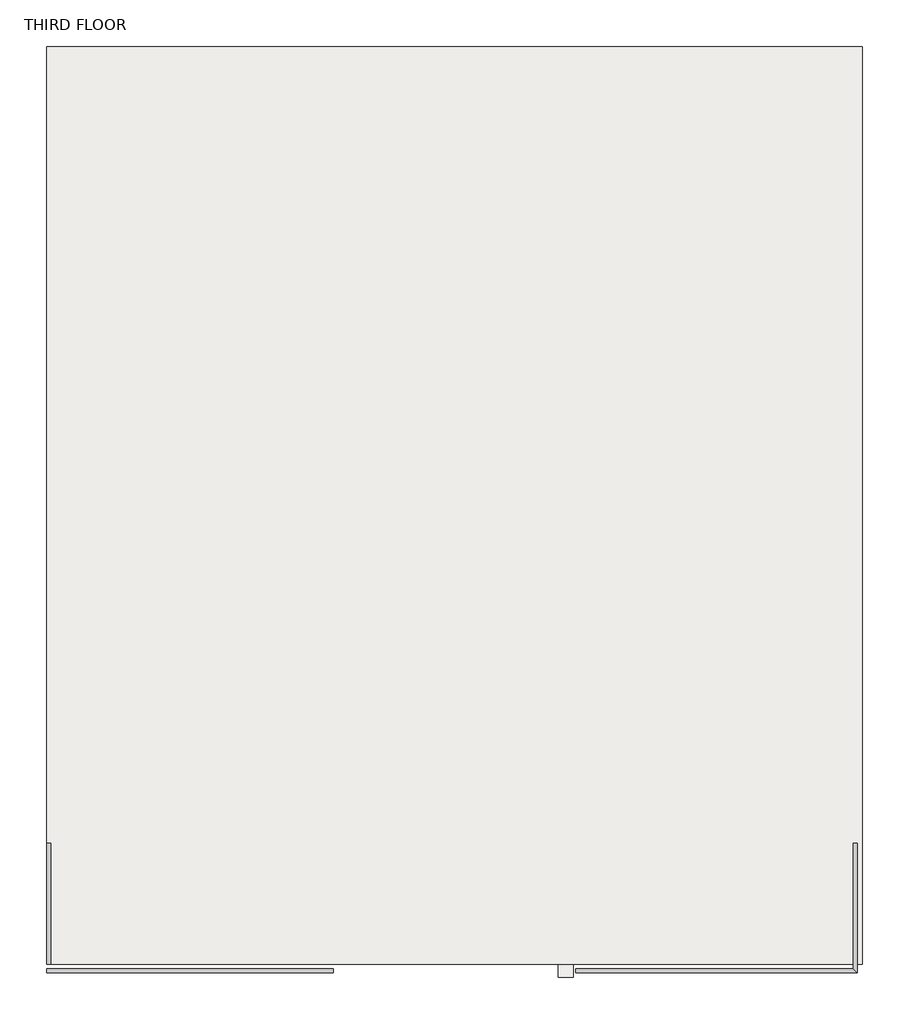
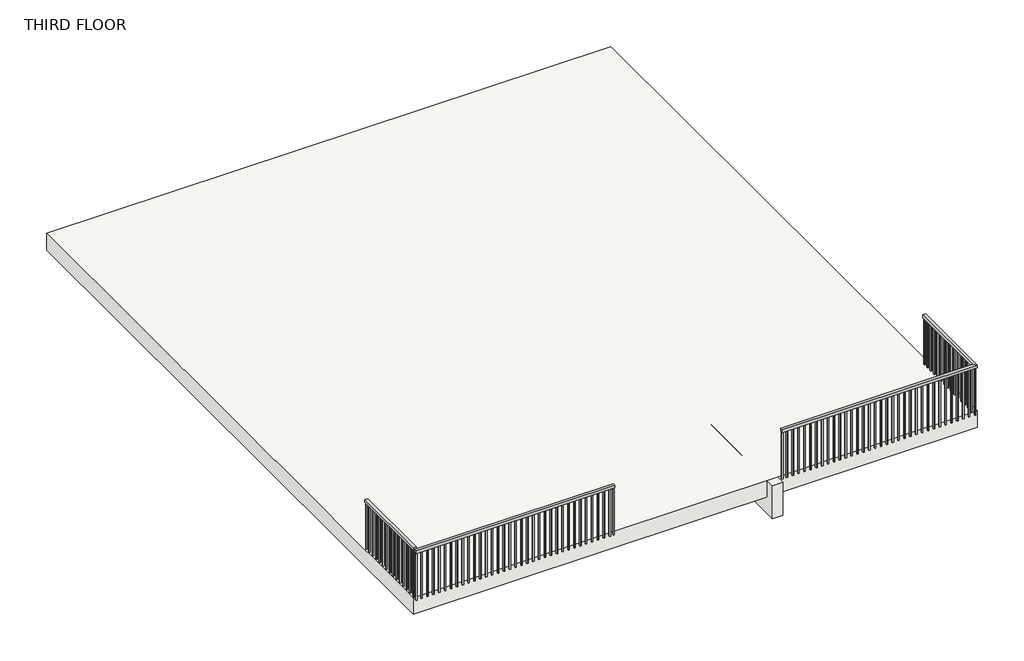
# One storey: 3 railings, 2 slabs.
"""IFC4 building model written with IfcOpenShell, lengths in millimetres."""

from ifc_helpers import new_model, si_unit, frame, origin, place, context, project, spatial, polyline, outline, extrude, faceted_brep, transform, mapped, element, save
from components import floors_4_floors_3_d07f1cc1

model = new_model("IFC4")

# Units and contexts
model_context = context("Model", 3, world=origin())
ifc_project = project(units=[si_unit("LENGTHUNIT", "METRE", prefix="MILLI")], contexts=[model_context])

# Site, building, storey
site = spatial("IfcSite", under=ifc_project)
building = spatial("IfcBuilding", under=site)
storey = spatial("IfcBuildingStorey", under=building, Name="THIRD FLOOR", Elevation=9144.0)

# Railings
placement = place(None, origin())
element("IfcRailing", 1, ObjectType="Handrail - Rectangular", at=placement, inside=storey, context=model_context, shape_type="SweptSolid", body=[
    extrude(outline(polyline([(-6322.0230786, -2172.0464178), (-6322.0230786, -2121.2464178), (-2893.0230786, -2121.2464178), (-2893.0230786, -2172.0464178), (-6322.0230786, -2172.0464178)])), frame((0.0, 0.0, 10007.6), z_axis=(0.0, 0.0, 1.0), x_axis=(1.0, 0.0, 0.0)), (0.0, 0.0, 1.0), 50.8),
    extrude(outline(polyline([(-2978.7480786, -2156.1714178), (-2978.7480786, -2137.1214178), (-2959.6980786, -2137.1214178), (-2959.6980786, -2156.1714178), (-2978.7480786, -2156.1714178)])), frame((0.0, 0.0, 9144.0), z_axis=(0.0, 0.0, 1.0), x_axis=(1.0, 0.0, 0.0)), (0.0, 0.0, 1.0), 863.6),
    extrude(outline(polyline([(-3080.3480786, -2156.1714178), (-3080.3480786, -2137.1214178), (-3061.2980786, -2137.1214178), (-3061.2980786, -2156.1714178), (-3080.3480786, -2156.1714178)])), frame((0.0, 0.0, 9144.0), z_axis=(0.0, 0.0, 1.0), x_axis=(1.0, 0.0, 0.0)), (0.0, 0.0, 1.0), 863.6),
    extrude(outline(polyline([(-3181.9480786, -2156.1714178), (-3181.9480786, -2137.1214178), (-3162.8980786, -2137.1214178), (-3162.8980786, -2156.1714178), (-3181.9480786, -2156.1714178)])), frame((0.0, 0.0, 9144.0), z_axis=(0.0, 0.0, 1.0), x_axis=(1.0, 0.0, 0.0)), (0.0, 0.0, 1.0), 863.6),
    extrude(outline(polyline([(-3283.5480786, -2156.1714178), (-3283.5480786, -2137.1214178), (-3264.4980786, -2137.1214178), (-3264.4980786, -2156.1714178), (-3283.5480786, -2156.1714178)])), frame((0.0, 0.0, 9144.0), z_axis=(0.0, 0.0, 1.0), x_axis=(1.0, 0.0, 0.0)), (0.0, 0.0, 1.0), 863.6),
    extrude(outline(polyline([(-3385.1480786, -2156.1714178), (-3385.1480786, -2137.1214178), (-3366.0980786, -2137.1214178), (-3366.0980786, -2156.1714178), (-3385.1480786, -2156.1714178)])), frame((0.0, 0.0, 9144.0), z_axis=(0.0, 0.0, 1.0), x_axis=(1.0, 0.0, 0.0)), (0.0, 0.0, 1.0), 863.6),
    extrude(outline(polyline([(-3486.7480786, -2156.1714178), (-3486.7480786, -2137.1214178), (-3467.6980786, -2137.1214178), (-3467.6980786, -2156.1714178), (-3486.7480786, -2156.1714178)])), frame((0.0, 0.0, 9144.0), z_axis=(0.0, 0.0, 1.0), x_axis=(1.0, 0.0, 0.0)), (0.0, 0.0, 1.0), 863.6),
    extrude(outline(polyline([(-3588.3480786, -2156.1714178), (-3588.3480786, -2137.1214178), (-3569.2980786, -2137.1214178), (-3569.2980786, -2156.1714178), (-3588.3480786, -2156.1714178)])), frame((0.0, 0.0, 9144.0), z_axis=(0.0, 0.0, 1.0), x_axis=(1.0, 0.0, 0.0)), (0.0, 0.0, 1.0), 863.6),
    extrude(outline(polyline([(-3689.9480786, -2156.1714178), (-3689.9480786, -2137.1214178), (-3670.8980786, -2137.1214178), (-3670.8980786, -2156.1714178), (-3689.9480786, -2156.1714178)])), frame((0.0, 0.0, 9144.0), z_axis=(0.0, 0.0, 1.0), x_axis=(1.0, 0.0, 0.0)), (0.0, 0.0, 1.0), 863.6),
    extrude(outline(polyline([(-3791.5480786, -2156.1714178), (-3791.5480786, -2137.1214178), (-3772.4980786, -2137.1214178), (-3772.4980786, -2156.1714178), (-3791.5480786, -2156.1714178)])), frame((0.0, 0.0, 9144.0), z_axis=(0.0, 0.0, 1.0), x_axis=(1.0, 0.0, 0.0)), (0.0, 0.0, 1.0), 863.6),
    extrude(outline(polyline([(-3893.1480786, -2156.1714178), (-3893.1480786, -2137.1214178), (-3874.0980786, -2137.1214178), (-3874.0980786, -2156.1714178), (-3893.1480786, -2156.1714178)])), frame((0.0, 0.0, 9144.0), z_axis=(0.0, 0.0, 1.0), x_axis=(1.0, 0.0, 0.0)), (0.0, 0.0, 1.0), 863.6),
    extrude(outline(polyline([(-3994.7480786, -2156.1714178), (-3994.7480786, -2137.1214178), (-3975.6980786, -2137.1214178), (-3975.6980786, -2156.1714178), (-3994.7480786, -2156.1714178)])), frame((0.0, 0.0, 9144.0), z_axis=(0.0, 0.0, 1.0), x_axis=(1.0, 0.0, 0.0)), (0.0, 0.0, 1.0), 863.6),
    extrude(outline(polyline([(-4096.3480786, -2156.1714178), (-4096.3480786, -2137.1214178), (-4077.2980786, -2137.1214178), (-4077.2980786, -2156.1714178), (-4096.3480786, -2156.1714178)])), frame((0.0, 0.0, 9144.0), z_axis=(0.0, 0.0, 1.0), x_axis=(1.0, 0.0, 0.0)), (0.0, 0.0, 1.0), 863.6),
    extrude(outline(polyline([(-4197.9480786, -2156.1714178), (-4197.9480786, -2137.1214178), (-4178.8980786, -2137.1214178), (-4178.8980786, -2156.1714178), (-4197.9480786, -2156.1714178)])), frame((0.0, 0.0, 9144.0), z_axis=(0.0, 0.0, 1.0), x_axis=(1.0, 0.0, 0.0)), (0.0, 0.0, 1.0), 863.6),
    extrude(outline(polyline([(-4299.5480786, -2156.1714178), (-4299.5480786, -2137.1214178), (-4280.4980786, -2137.1214178), (-4280.4980786, -2156.1714178), (-4299.5480786, -2156.1714178)])), frame((0.0, 0.0, 9144.0), z_axis=(0.0, 0.0, 1.0), x_axis=(1.0, 0.0, 0.0)), (0.0, 0.0, 1.0), 863.6),
    extrude(outline(polyline([(-4401.1480786, -2156.1714178), (-4401.1480786, -2137.1214178), (-4382.0980786, -2137.1214178), (-4382.0980786, -2156.1714178), (-4401.1480786, -2156.1714178)])), frame((0.0, 0.0, 9144.0), z_axis=(0.0, 0.0, 1.0), x_axis=(1.0, 0.0, 0.0)), (0.0, 0.0, 1.0), 863.6),
    extrude(outline(polyline([(-4502.7480786, -2156.1714178), (-4502.7480786, -2137.1214178), (-4483.6980786, -2137.1214178), (-4483.6980786, -2156.1714178), (-4502.7480786, -2156.1714178)])), frame((0.0, 0.0, 9144.0), z_axis=(0.0, 0.0, 1.0), x_axis=(1.0, 0.0, 0.0)), (0.0, 0.0, 1.0), 863.6),
    extrude(outline(polyline([(-4604.3480786, -2156.1714178), (-4604.3480786, -2137.1214178), (-4585.2980786, -2137.1214178), (-4585.2980786, -2156.1714178), (-4604.3480786, -2156.1714178)])), frame((0.0, 0.0, 9144.0), z_axis=(0.0, 0.0, 1.0), x_axis=(1.0, 0.0, 0.0)), (0.0, 0.0, 1.0), 863.6),
    extrude(outline(polyline([(-4705.9480786, -2156.1714178), (-4705.9480786, -2137.1214178), (-4686.8980786, -2137.1214178), (-4686.8980786, -2156.1714178), (-4705.9480786, -2156.1714178)])), frame((0.0, 0.0, 9144.0), z_axis=(0.0, 0.0, 1.0), x_axis=(1.0, 0.0, 0.0)), (0.0, 0.0, 1.0), 863.6),
    extrude(outline(polyline([(-4807.5480786, -2156.1714178), (-4807.5480786, -2137.1214178), (-4788.4980786, -2137.1214178), (-4788.4980786, -2156.1714178), (-4807.5480786, -2156.1714178)])), frame((0.0, 0.0, 9144.0), z_axis=(0.0, 0.0, 1.0), x_axis=(1.0, 0.0, 0.0)), (0.0, 0.0, 1.0), 863.6),
    extrude(outline(polyline([(-4909.1480786, -2156.1714178), (-4909.1480786, -2137.1214178), (-4890.0980786, -2137.1214178), (-4890.0980786, -2156.1714178), (-4909.1480786, -2156.1714178)])), frame((0.0, 0.0, 9144.0), z_axis=(0.0, 0.0, 1.0), x_axis=(1.0, 0.0, 0.0)), (0.0, 0.0, 1.0), 863.6),
    extrude(outline(polyline([(-5010.7480786, -2156.1714178), (-5010.7480786, -2137.1214178), (-4991.6980786, -2137.1214178), (-4991.6980786, -2156.1714178), (-5010.7480786, -2156.1714178)])), frame((0.0, 0.0, 9144.0), z_axis=(0.0, 0.0, 1.0), x_axis=(1.0, 0.0, 0.0)), (0.0, 0.0, 1.0), 863.6),
    extrude(outline(polyline([(-5112.3480786, -2156.1714178), (-5112.3480786, -2137.1214178), (-5093.2980786, -2137.1214178), (-5093.2980786, -2156.1714178), (-5112.3480786, -2156.1714178)])), frame((0.0, 0.0, 9144.0), z_axis=(0.0, 0.0, 1.0), x_axis=(1.0, 0.0, 0.0)), (0.0, 0.0, 1.0), 863.6),
    extrude(outline(polyline([(-5213.9480786, -2156.1714178), (-5213.9480786, -2137.1214178), (-5194.8980786, -2137.1214178), (-5194.8980786, -2156.1714178), (-5213.9480786, -2156.1714178)])), frame((0.0, 0.0, 9144.0), z_axis=(0.0, 0.0, 1.0), x_axis=(1.0, 0.0, 0.0)), (0.0, 0.0, 1.0), 863.6),
    extrude(outline(polyline([(-5315.5480786, -2156.1714178), (-5315.5480786, -2137.1214178), (-5296.4980786, -2137.1214178), (-5296.4980786, -2156.1714178), (-5315.5480786, -2156.1714178)])), frame((0.0, 0.0, 9144.0), z_axis=(0.0, 0.0, 1.0), x_axis=(1.0, 0.0, 0.0)), (0.0, 0.0, 1.0), 863.6),
    extrude(outline(polyline([(-5417.1480786, -2156.1714178), (-5417.1480786, -2137.1214178), (-5398.0980786, -2137.1214178), (-5398.0980786, -2156.1714178), (-5417.1480786, -2156.1714178)])), frame((0.0, 0.0, 9144.0), z_axis=(0.0, 0.0, 1.0), x_axis=(1.0, 0.0, 0.0)), (0.0, 0.0, 1.0), 863.6),
    extrude(outline(polyline([(-5518.7480786, -2156.1714178), (-5518.7480786, -2137.1214178), (-5499.6980786, -2137.1214178), (-5499.6980786, -2156.1714178), (-5518.7480786, -2156.1714178)])), frame((0.0, 0.0, 9144.0), z_axis=(0.0, 0.0, 1.0), x_axis=(1.0, 0.0, 0.0)), (0.0, 0.0, 1.0), 863.6),
    extrude(outline(polyline([(-5620.3480786, -2156.1714178), (-5620.3480786, -2137.1214178), (-5601.2980786, -2137.1214178), (-5601.2980786, -2156.1714178), (-5620.3480786, -2156.1714178)])), frame((0.0, 0.0, 9144.0), z_axis=(0.0, 0.0, 1.0), x_axis=(1.0, 0.0, 0.0)), (0.0, 0.0, 1.0), 863.6),
    extrude(outline(polyline([(-5721.9480786, -2156.1714178), (-5721.9480786, -2137.1214178), (-5702.8980786, -2137.1214178), (-5702.8980786, -2156.1714178), (-5721.9480786, -2156.1714178)])), frame((0.0, 0.0, 9144.0), z_axis=(0.0, 0.0, 1.0), x_axis=(1.0, 0.0, 0.0)), (0.0, 0.0, 1.0), 863.6),
    extrude(outline(polyline([(-5823.5480786, -2156.1714178), (-5823.5480786, -2137.1214178), (-5804.4980786, -2137.1214178), (-5804.4980786, -2156.1714178), (-5823.5480786, -2156.1714178)])), frame((0.0, 0.0, 9144.0), z_axis=(0.0, 0.0, 1.0), x_axis=(1.0, 0.0, 0.0)), (0.0, 0.0, 1.0), 863.6),
    extrude(outline(polyline([(-5925.1480786, -2156.1714178), (-5925.1480786, -2137.1214178), (-5906.0980786, -2137.1214178), (-5906.0980786, -2156.1714178), (-5925.1480786, -2156.1714178)])), frame((0.0, 0.0, 9144.0), z_axis=(0.0, 0.0, 1.0), x_axis=(1.0, 0.0, 0.0)), (0.0, 0.0, 1.0), 863.6),
    extrude(outline(polyline([(-6026.7480786, -2156.1714178), (-6026.7480786, -2137.1214178), (-6007.6980786, -2137.1214178), (-6007.6980786, -2156.1714178), (-6026.7480786, -2156.1714178)])), frame((0.0, 0.0, 9144.0), z_axis=(0.0, 0.0, 1.0), x_axis=(1.0, 0.0, 0.0)), (0.0, 0.0, 1.0), 863.6),
    extrude(outline(polyline([(-6128.3480786, -2156.1714178), (-6128.3480786, -2137.1214178), (-6109.2980786, -2137.1214178), (-6109.2980786, -2156.1714178), (-6128.3480786, -2156.1714178)])), frame((0.0, 0.0, 9144.0), z_axis=(0.0, 0.0, 1.0), x_axis=(1.0, 0.0, 0.0)), (0.0, 0.0, 1.0), 863.6),
    extrude(outline(polyline([(-6229.9480786, -2156.1714178), (-6229.9480786, -2137.1214178), (-6210.8980786, -2137.1214178), (-6210.8980786, -2156.1714178), (-6229.9480786, -2156.1714178)])), frame((0.0, 0.0, 9144.0), z_axis=(0.0, 0.0, 1.0), x_axis=(1.0, 0.0, 0.0)), (0.0, 0.0, 1.0), 863.6),
    extrude(outline(polyline([(-2912.0730786, -2156.1714178), (-2912.0730786, -2137.1214178), (-2893.0230786, -2137.1214178), (-2893.0230786, -2156.1714178), (-2912.0730786, -2156.1714178)])), frame((0.0, 0.0, 9144.0), z_axis=(0.0, 0.0, 1.0), x_axis=(1.0, 0.0, 0.0)), (0.0, 0.0, 1.0), 863.6),
    extrude(outline(polyline([(-6322.0230786, -2156.1714178), (-6322.0230786, -2137.1214178), (-6302.9730786, -2137.1214178), (-6302.9730786, -2156.1714178), (-6322.0230786, -2156.1714178)])), frame((0.0, 0.0, 9144.0), z_axis=(0.0, 0.0, 1.0), x_axis=(1.0, 0.0, 0.0)), (0.0, 0.0, 1.0), 863.6),
])
element("IfcRailing", 2, ObjectType="Handrail - Rectangular", at=placement, inside=storey, context=model_context, shape_type="SolidModel", body=[
    faceted_brep([(3370.3245405, -622.6464931, 10058.4), (3370.3245405, -622.6464931, 10007.6), (3319.5245405, -622.6464931, 10007.6), (3319.5245405, -622.6464931, 10058.4), (3370.3245405, -2172.0464178, 10058.4), (3370.3245405, -2172.0464178, 10007.6), (3319.5245405, -2121.2464178, 10007.6), (3319.5245405, -2121.2464178, 10058.4), (2.5769214, -2172.0464178, 10058.4), (2.5769214, -2121.2464178, 10058.4), (2.5769214, -2121.2464178, 10007.6), (2.5769214, -2172.0464178, 10007.6)], [[[0, 1, 2, 3]], [[1, 0, 4, 5]], [[2, 1, 5, 6]], [[3, 2, 6, 7]], [[0, 3, 7, 4]], [[8, 9, 10, 11]], [[5, 4, 8, 11]], [[6, 5, 11, 10]], [[7, 6, 10, 9]], [[4, 7, 9, 8]]]),
    extrude(outline(polyline([(103.2495405, -2137.1214178), (103.2495405, -2156.1714178), (84.1995405, -2156.1714178), (84.1995405, -2137.1214178), (103.2495405, -2137.1214178)])), frame((0.0, 0.0, 9144.0), z_axis=(0.0, 0.0, 1.0), x_axis=(1.0, 0.0, 0.0)), (0.0, 0.0, 1.0), 863.6),
    extrude(outline(polyline([(204.8495405, -2137.1214178), (204.8495405, -2156.1714178), (185.7995405, -2156.1714178), (185.7995405, -2137.1214178), (204.8495405, -2137.1214178)])), frame((0.0, 0.0, 9144.0), z_axis=(0.0, 0.0, 1.0), x_axis=(1.0, 0.0, 0.0)), (0.0, 0.0, 1.0), 863.6),
    extrude(outline(polyline([(306.4495405, -2137.1214178), (306.4495405, -2156.1714178), (287.3995405, -2156.1714178), (287.3995405, -2137.1214178), (306.4495405, -2137.1214178)])), frame((0.0, 0.0, 9144.0), z_axis=(0.0, 0.0, 1.0), x_axis=(1.0, 0.0, 0.0)), (0.0, 0.0, 1.0), 863.6),
    extrude(outline(polyline([(408.0495405, -2137.1214178), (408.0495405, -2156.1714178), (388.9995405, -2156.1714178), (388.9995405, -2137.1214178), (408.0495405, -2137.1214178)])), frame((0.0, 0.0, 9144.0), z_axis=(0.0, 0.0, 1.0), x_axis=(1.0, 0.0, 0.0)), (0.0, 0.0, 1.0), 863.6),
    extrude(outline(polyline([(509.6495405, -2137.1214178), (509.6495405, -2156.1714178), (490.5995405, -2156.1714178), (490.5995405, -2137.1214178), (509.6495405, -2137.1214178)])), frame((0.0, 0.0, 9144.0), z_axis=(0.0, 0.0, 1.0), x_axis=(1.0, 0.0, 0.0)), (0.0, 0.0, 1.0), 863.6),
    extrude(outline(polyline([(611.2495405, -2137.1214178), (611.2495405, -2156.1714178), (592.1995405, -2156.1714178), (592.1995405, -2137.1214178), (611.2495405, -2137.1214178)])), frame((0.0, 0.0, 9144.0), z_axis=(0.0, 0.0, 1.0), x_axis=(1.0, 0.0, 0.0)), (0.0, 0.0, 1.0), 863.6),
    extrude(outline(polyline([(712.8495405, -2137.1214178), (712.8495405, -2156.1714178), (693.7995405, -2156.1714178), (693.7995405, -2137.1214178), (712.8495405, -2137.1214178)])), frame((0.0, 0.0, 9144.0), z_axis=(0.0, 0.0, 1.0), x_axis=(1.0, 0.0, 0.0)), (0.0, 0.0, 1.0), 863.6),
    extrude(outline(polyline([(814.4495405, -2137.1214178), (814.4495405, -2156.1714178), (795.3995405, -2156.1714178), (795.3995405, -2137.1214178), (814.4495405, -2137.1214178)])), frame((0.0, 0.0, 9144.0), z_axis=(0.0, 0.0, 1.0), x_axis=(1.0, 0.0, 0.0)), (0.0, 0.0, 1.0), 863.6),
    extrude(outline(polyline([(916.0495405, -2137.1214178), (916.0495405, -2156.1714178), (896.9995405, -2156.1714178), (896.9995405, -2137.1214178), (916.0495405, -2137.1214178)])), frame((0.0, 0.0, 9144.0), z_axis=(0.0, 0.0, 1.0), x_axis=(1.0, 0.0, 0.0)), (0.0, 0.0, 1.0), 863.6),
    extrude(outline(polyline([(1017.6495405, -2137.1214178), (1017.6495405, -2156.1714178), (998.5995405, -2156.1714178), (998.5995405, -2137.1214178), (1017.6495405, -2137.1214178)])), frame((0.0, 0.0, 9144.0), z_axis=(0.0, 0.0, 1.0), x_axis=(1.0, 0.0, 0.0)), (0.0, 0.0, 1.0), 863.6),
    extrude(outline(polyline([(1119.2495405, -2137.1214178), (1119.2495405, -2156.1714178), (1100.1995405, -2156.1714178), (1100.1995405, -2137.1214178), (1119.2495405, -2137.1214178)])), frame((0.0, 0.0, 9144.0), z_axis=(0.0, 0.0, 1.0), x_axis=(1.0, 0.0, 0.0)), (0.0, 0.0, 1.0), 863.6),
    extrude(outline(polyline([(1220.8495405, -2137.1214178), (1220.8495405, -2156.1714178), (1201.7995405, -2156.1714178), (1201.7995405, -2137.1214178), (1220.8495405, -2137.1214178)])), frame((0.0, 0.0, 9144.0), z_axis=(0.0, 0.0, 1.0), x_axis=(1.0, 0.0, 0.0)), (0.0, 0.0, 1.0), 863.6),
    extrude(outline(polyline([(1322.4495405, -2137.1214178), (1322.4495405, -2156.1714178), (1303.3995405, -2156.1714178), (1303.3995405, -2137.1214178), (1322.4495405, -2137.1214178)])), frame((0.0, 0.0, 9144.0), z_axis=(0.0, 0.0, 1.0), x_axis=(1.0, 0.0, 0.0)), (0.0, 0.0, 1.0), 863.6),
    extrude(outline(polyline([(1424.0495405, -2137.1214178), (1424.0495405, -2156.1714178), (1404.9995405, -2156.1714178), (1404.9995405, -2137.1214178), (1424.0495405, -2137.1214178)])), frame((0.0, 0.0, 9144.0), z_axis=(0.0, 0.0, 1.0), x_axis=(1.0, 0.0, 0.0)), (0.0, 0.0, 1.0), 863.6),
    extrude(outline(polyline([(1525.6495405, -2137.1214178), (1525.6495405, -2156.1714178), (1506.5995405, -2156.1714178), (1506.5995405, -2137.1214178), (1525.6495405, -2137.1214178)])), frame((0.0, 0.0, 9144.0), z_axis=(0.0, 0.0, 1.0), x_axis=(1.0, 0.0, 0.0)), (0.0, 0.0, 1.0), 863.6),
    extrude(outline(polyline([(1627.2495405, -2137.1214178), (1627.2495405, -2156.1714178), (1608.1995405, -2156.1714178), (1608.1995405, -2137.1214178), (1627.2495405, -2137.1214178)])), frame((0.0, 0.0, 9144.0), z_axis=(0.0, 0.0, 1.0), x_axis=(1.0, 0.0, 0.0)), (0.0, 0.0, 1.0), 863.6),
    extrude(outline(polyline([(1728.8495405, -2137.1214178), (1728.8495405, -2156.1714178), (1709.7995405, -2156.1714178), (1709.7995405, -2137.1214178), (1728.8495405, -2137.1214178)])), frame((0.0, 0.0, 9144.0), z_axis=(0.0, 0.0, 1.0), x_axis=(1.0, 0.0, 0.0)), (0.0, 0.0, 1.0), 863.6),
    extrude(outline(polyline([(1830.4495405, -2137.1214178), (1830.4495405, -2156.1714178), (1811.3995405, -2156.1714178), (1811.3995405, -2137.1214178), (1830.4495405, -2137.1214178)])), frame((0.0, 0.0, 9144.0), z_axis=(0.0, 0.0, 1.0), x_axis=(1.0, 0.0, 0.0)), (0.0, 0.0, 1.0), 863.6),
    extrude(outline(polyline([(1932.0495405, -2137.1214178), (1932.0495405, -2156.1714178), (1912.9995405, -2156.1714178), (1912.9995405, -2137.1214178), (1932.0495405, -2137.1214178)])), frame((0.0, 0.0, 9144.0), z_axis=(0.0, 0.0, 1.0), x_axis=(1.0, 0.0, 0.0)), (0.0, 0.0, 1.0), 863.6),
    extrude(outline(polyline([(2033.6495405, -2137.1214178), (2033.6495405, -2156.1714178), (2014.5995405, -2156.1714178), (2014.5995405, -2137.1214178), (2033.6495405, -2137.1214178)])), frame((0.0, 0.0, 9144.0), z_axis=(0.0, 0.0, 1.0), x_axis=(1.0, 0.0, 0.0)), (0.0, 0.0, 1.0), 863.6),
    extrude(outline(polyline([(2135.2495405, -2137.1214178), (2135.2495405, -2156.1714178), (2116.1995405, -2156.1714178), (2116.1995405, -2137.1214178), (2135.2495405, -2137.1214178)])), frame((0.0, 0.0, 9144.0), z_axis=(0.0, 0.0, 1.0), x_axis=(1.0, 0.0, 0.0)), (0.0, 0.0, 1.0), 863.6),
    extrude(outline(polyline([(2236.8495405, -2137.1214178), (2236.8495405, -2156.1714178), (2217.7995405, -2156.1714178), (2217.7995405, -2137.1214178), (2236.8495405, -2137.1214178)])), frame((0.0, 0.0, 9144.0), z_axis=(0.0, 0.0, 1.0), x_axis=(1.0, 0.0, 0.0)), (0.0, 0.0, 1.0), 863.6),
    extrude(outline(polyline([(2338.4495405, -2137.1214178), (2338.4495405, -2156.1714178), (2319.3995405, -2156.1714178), (2319.3995405, -2137.1214178), (2338.4495405, -2137.1214178)])), frame((0.0, 0.0, 9144.0), z_axis=(0.0, 0.0, 1.0), x_axis=(1.0, 0.0, 0.0)), (0.0, 0.0, 1.0), 863.6),
    extrude(outline(polyline([(2440.0495405, -2137.1214178), (2440.0495405, -2156.1714178), (2420.9995405, -2156.1714178), (2420.9995405, -2137.1214178), (2440.0495405, -2137.1214178)])), frame((0.0, 0.0, 9144.0), z_axis=(0.0, 0.0, 1.0), x_axis=(1.0, 0.0, 0.0)), (0.0, 0.0, 1.0), 863.6),
    extrude(outline(polyline([(2541.6495405, -2137.1214178), (2541.6495405, -2156.1714178), (2522.5995405, -2156.1714178), (2522.5995405, -2137.1214178), (2541.6495405, -2137.1214178)])), frame((0.0, 0.0, 9144.0), z_axis=(0.0, 0.0, 1.0), x_axis=(1.0, 0.0, 0.0)), (0.0, 0.0, 1.0), 863.6),
    extrude(outline(polyline([(2643.2495405, -2137.1214178), (2643.2495405, -2156.1714178), (2624.1995405, -2156.1714178), (2624.1995405, -2137.1214178), (2643.2495405, -2137.1214178)])), frame((0.0, 0.0, 9144.0), z_axis=(0.0, 0.0, 1.0), x_axis=(1.0, 0.0, 0.0)), (0.0, 0.0, 1.0), 863.6),
    extrude(outline(polyline([(2744.8495405, -2137.1214178), (2744.8495405, -2156.1714178), (2725.7995405, -2156.1714178), (2725.7995405, -2137.1214178), (2744.8495405, -2137.1214178)])), frame((0.0, 0.0, 9144.0), z_axis=(0.0, 0.0, 1.0), x_axis=(1.0, 0.0, 0.0)), (0.0, 0.0, 1.0), 863.6),
    extrude(outline(polyline([(2846.4495405, -2137.1214178), (2846.4495405, -2156.1714178), (2827.3995405, -2156.1714178), (2827.3995405, -2137.1214178), (2846.4495405, -2137.1214178)])), frame((0.0, 0.0, 9144.0), z_axis=(0.0, 0.0, 1.0), x_axis=(1.0, 0.0, 0.0)), (0.0, 0.0, 1.0), 863.6),
    extrude(outline(polyline([(2948.0495405, -2137.1214178), (2948.0495405, -2156.1714178), (2928.9995405, -2156.1714178), (2928.9995405, -2137.1214178), (2948.0495405, -2137.1214178)])), frame((0.0, 0.0, 9144.0), z_axis=(0.0, 0.0, 1.0), x_axis=(1.0, 0.0, 0.0)), (0.0, 0.0, 1.0), 863.6),
    extrude(outline(polyline([(3049.6495405, -2137.1214178), (3049.6495405, -2156.1714178), (3030.5995405, -2156.1714178), (3030.5995405, -2137.1214178), (3049.6495405, -2137.1214178)])), frame((0.0, 0.0, 9144.0), z_axis=(0.0, 0.0, 1.0), x_axis=(1.0, 0.0, 0.0)), (0.0, 0.0, 1.0), 863.6),
    extrude(outline(polyline([(3151.2495405, -2137.1214178), (3151.2495405, -2156.1714178), (3132.1995405, -2156.1714178), (3132.1995405, -2137.1214178), (3151.2495405, -2137.1214178)])), frame((0.0, 0.0, 9144.0), z_axis=(0.0, 0.0, 1.0), x_axis=(1.0, 0.0, 0.0)), (0.0, 0.0, 1.0), 863.6),
    extrude(outline(polyline([(3252.8495405, -2137.1214178), (3252.8495405, -2156.1714178), (3233.7995405, -2156.1714178), (3233.7995405, -2137.1214178), (3252.8495405, -2137.1214178)])), frame((0.0, 0.0, 9144.0), z_axis=(0.0, 0.0, 1.0), x_axis=(1.0, 0.0, 0.0)), (0.0, 0.0, 1.0), 863.6),
    extrude(outline(polyline([(3335.3995405, -2035.5214931), (3354.4495405, -2035.5214931), (3354.4495405, -2054.5714931), (3335.3995405, -2054.5714931), (3335.3995405, -2035.5214931)])), frame((0.0, 0.0, 9144.0), z_axis=(0.0, 0.0, 1.0), x_axis=(1.0, 0.0, 0.0)), (0.0, 0.0, 1.0), 863.6),
    extrude(outline(polyline([(3335.3995405, -1933.9214931), (3354.4495405, -1933.9214931), (3354.4495405, -1952.9714931), (3335.3995405, -1952.9714931), (3335.3995405, -1933.9214931)])), frame((0.0, 0.0, 9144.0), z_axis=(0.0, 0.0, 1.0), x_axis=(1.0, 0.0, 0.0)), (0.0, 0.0, 1.0), 863.6),
    extrude(outline(polyline([(3335.3995405, -1832.3214931), (3354.4495405, -1832.3214931), (3354.4495405, -1851.3714931), (3335.3995405, -1851.3714931), (3335.3995405, -1832.3214931)])), frame((0.0, 0.0, 9144.0), z_axis=(0.0, 0.0, 1.0), x_axis=(1.0, 0.0, 0.0)), (0.0, 0.0, 1.0), 863.6),
    extrude(outline(polyline([(3335.3995405, -1730.7214931), (3354.4495405, -1730.7214931), (3354.4495405, -1749.7714931), (3335.3995405, -1749.7714931), (3335.3995405, -1730.7214931)])), frame((0.0, 0.0, 9144.0), z_axis=(0.0, 0.0, 1.0), x_axis=(1.0, 0.0, 0.0)), (0.0, 0.0, 1.0), 863.6),
    extrude(outline(polyline([(3335.3995405, -1629.1214931), (3354.4495405, -1629.1214931), (3354.4495405, -1648.1714931), (3335.3995405, -1648.1714931), (3335.3995405, -1629.1214931)])), frame((0.0, 0.0, 9144.0), z_axis=(0.0, 0.0, 1.0), x_axis=(1.0, 0.0, 0.0)), (0.0, 0.0, 1.0), 863.6),
    extrude(outline(polyline([(3335.3995405, -1527.5214931), (3354.4495405, -1527.5214931), (3354.4495405, -1546.5714931), (3335.3995405, -1546.5714931), (3335.3995405, -1527.5214931)])), frame((0.0, 0.0, 9144.0), z_axis=(0.0, 0.0, 1.0), x_axis=(1.0, 0.0, 0.0)), (0.0, 0.0, 1.0), 863.6),
    extrude(outline(polyline([(3335.3995405, -1425.9214931), (3354.4495405, -1425.9214931), (3354.4495405, -1444.9714931), (3335.3995405, -1444.9714931), (3335.3995405, -1425.9214931)])), frame((0.0, 0.0, 9144.0), z_axis=(0.0, 0.0, 1.0), x_axis=(1.0, 0.0, 0.0)), (0.0, 0.0, 1.0), 863.6),
    extrude(outline(polyline([(3335.3995405, -1324.3214931), (3354.4495405, -1324.3214931), (3354.4495405, -1343.3714931), (3335.3995405, -1343.3714931), (3335.3995405, -1324.3214931)])), frame((0.0, 0.0, 9144.0), z_axis=(0.0, 0.0, 1.0), x_axis=(1.0, 0.0, 0.0)), (0.0, 0.0, 1.0), 863.6),
    extrude(outline(polyline([(3335.3995405, -1222.7214931), (3354.4495405, -1222.7214931), (3354.4495405, -1241.7714931), (3335.3995405, -1241.7714931), (3335.3995405, -1222.7214931)])), frame((0.0, 0.0, 9144.0), z_axis=(0.0, 0.0, 1.0), x_axis=(1.0, 0.0, 0.0)), (0.0, 0.0, 1.0), 863.6),
    extrude(outline(polyline([(3335.3995405, -1121.1214931), (3354.4495405, -1121.1214931), (3354.4495405, -1140.1714931), (3335.3995405, -1140.1714931), (3335.3995405, -1121.1214931)])), frame((0.0, 0.0, 9144.0), z_axis=(0.0, 0.0, 1.0), x_axis=(1.0, 0.0, 0.0)), (0.0, 0.0, 1.0), 863.6),
    extrude(outline(polyline([(3335.3995405, -1019.5214931), (3354.4495405, -1019.5214931), (3354.4495405, -1038.5714931), (3335.3995405, -1038.5714931), (3335.3995405, -1019.5214931)])), frame((0.0, 0.0, 9144.0), z_axis=(0.0, 0.0, 1.0), x_axis=(1.0, 0.0, 0.0)), (0.0, 0.0, 1.0), 863.6),
    extrude(outline(polyline([(3335.3995405, -917.9214931), (3354.4495405, -917.9214931), (3354.4495405, -936.9714931), (3335.3995405, -936.9714931), (3335.3995405, -917.9214931)])), frame((0.0, 0.0, 9144.0), z_axis=(0.0, 0.0, 1.0), x_axis=(1.0, 0.0, 0.0)), (0.0, 0.0, 1.0), 863.6),
    extrude(outline(polyline([(3335.3995405, -816.3214931), (3354.4495405, -816.3214931), (3354.4495405, -835.3714931), (3335.3995405, -835.3714931), (3335.3995405, -816.3214931)])), frame((0.0, 0.0, 9144.0), z_axis=(0.0, 0.0, 1.0), x_axis=(1.0, 0.0, 0.0)), (0.0, 0.0, 1.0), 863.6),
    extrude(outline(polyline([(3335.3995405, -714.7214931), (3354.4495405, -714.7214931), (3354.4495405, -733.7714931), (3335.3995405, -733.7714931), (3335.3995405, -714.7214931)])), frame((0.0, 0.0, 9144.0), z_axis=(0.0, 0.0, 1.0), x_axis=(1.0, 0.0, 0.0)), (0.0, 0.0, 1.0), 863.6),
    extrude(outline(polyline([(3335.3995405, -2137.1214178), (3354.4495405, -2137.1214178), (3354.4495405, -2156.1714178), (3335.3995405, -2156.1714178), (3335.3995405, -2137.1214178)])), frame((0.0, 0.0, 9144.0), z_axis=(0.0, 0.0, 1.0), x_axis=(1.0, 0.0, 0.0)), (0.0, 0.0, 1.0), 863.6),
    extrude(outline(polyline([(21.6269214, -2137.1214178), (21.6269214, -2156.1714178), (2.5769214, -2156.1714178), (2.5769214, -2137.1214178), (21.6269214, -2137.1214178)])), frame((0.0, 0.0, 9144.0), z_axis=(0.0, 0.0, 1.0), x_axis=(1.0, 0.0, 0.0)), (0.0, 0.0, 1.0), 863.6),
    extrude(outline(polyline([(3335.3995405, -622.6464931), (3354.4495405, -622.6464931), (3354.4495405, -641.6964931), (3335.3995405, -641.6964931), (3335.3995405, -622.6464931)])), frame((0.0, 0.0, 9144.0), z_axis=(0.0, 0.0, 1.0), x_axis=(1.0, 0.0, 0.0)), (0.0, 0.0, 1.0), 863.6),
])
element("IfcRailing", 3, ObjectType="Handrail - Rectangular", at=placement, inside=storey, context=model_context, shape_type="SweptSolid", body=[
    extrude(outline(polyline([(-6322.0230786, -622.6464931), (-6271.2230786, -622.6464931), (-6271.2230786, -2070.4464178), (-6322.0230786, -2070.4464178), (-6322.0230786, -622.6464931)])), frame((0.0, 0.0, 10007.6), z_axis=(0.0, 0.0, 1.0), x_axis=(1.0, 0.0, 0.0)), (0.0, 0.0, 1.0), 50.8),
    extrude(outline(polyline([(-6306.1480786, -2035.5214931), (-6287.0980786, -2035.5214931), (-6287.0980786, -2054.5714931), (-6306.1480786, -2054.5714931), (-6306.1480786, -2035.5214931)])), frame((0.0, 0.0, 9144.0), z_axis=(0.0, 0.0, 1.0), x_axis=(1.0, 0.0, 0.0)), (0.0, 0.0, 1.0), 863.6),
    extrude(outline(polyline([(-6306.1480786, -1933.9214931), (-6287.0980786, -1933.9214931), (-6287.0980786, -1952.9714931), (-6306.1480786, -1952.9714931), (-6306.1480786, -1933.9214931)])), frame((0.0, 0.0, 9144.0), z_axis=(0.0, 0.0, 1.0), x_axis=(1.0, 0.0, 0.0)), (0.0, 0.0, 1.0), 863.6),
    extrude(outline(polyline([(-6306.1480786, -1832.3214931), (-6287.0980786, -1832.3214931), (-6287.0980786, -1851.3714931), (-6306.1480786, -1851.3714931), (-6306.1480786, -1832.3214931)])), frame((0.0, 0.0, 9144.0), z_axis=(0.0, 0.0, 1.0), x_axis=(1.0, 0.0, 0.0)), (0.0, 0.0, 1.0), 863.6),
    extrude(outline(polyline([(-6306.1480786, -1730.7214931), (-6287.0980786, -1730.7214931), (-6287.0980786, -1749.7714931), (-6306.1480786, -1749.7714931), (-6306.1480786, -1730.7214931)])), frame((0.0, 0.0, 9144.0), z_axis=(0.0, 0.0, 1.0), x_axis=(1.0, 0.0, 0.0)), (0.0, 0.0, 1.0), 863.6),
    extrude(outline(polyline([(-6306.1480786, -1629.1214931), (-6287.0980786, -1629.1214931), (-6287.0980786, -1648.1714931), (-6306.1480786, -1648.1714931), (-6306.1480786, -1629.1214931)])), frame((0.0, 0.0, 9144.0), z_axis=(0.0, 0.0, 1.0), x_axis=(1.0, 0.0, 0.0)), (0.0, 0.0, 1.0), 863.6),
    extrude(outline(polyline([(-6306.1480786, -1527.5214931), (-6287.0980786, -1527.5214931), (-6287.0980786, -1546.5714931), (-6306.1480786, -1546.5714931), (-6306.1480786, -1527.5214931)])), frame((0.0, 0.0, 9144.0), z_axis=(0.0, 0.0, 1.0), x_axis=(1.0, 0.0, 0.0)), (0.0, 0.0, 1.0), 863.6),
    extrude(outline(polyline([(-6306.1480786, -1425.9214931), (-6287.0980786, -1425.9214931), (-6287.0980786, -1444.9714931), (-6306.1480786, -1444.9714931), (-6306.1480786, -1425.9214931)])), frame((0.0, 0.0, 9144.0), z_axis=(0.0, 0.0, 1.0), x_axis=(1.0, 0.0, 0.0)), (0.0, 0.0, 1.0), 863.6),
    extrude(outline(polyline([(-6306.1480786, -1324.3214931), (-6287.0980786, -1324.3214931), (-6287.0980786, -1343.3714931), (-6306.1480786, -1343.3714931), (-6306.1480786, -1324.3214931)])), frame((0.0, 0.0, 9144.0), z_axis=(0.0, 0.0, 1.0), x_axis=(1.0, 0.0, 0.0)), (0.0, 0.0, 1.0), 863.6),
    extrude(outline(polyline([(-6306.1480786, -1222.7214931), (-6287.0980786, -1222.7214931), (-6287.0980786, -1241.7714931), (-6306.1480786, -1241.7714931), (-6306.1480786, -1222.7214931)])), frame((0.0, 0.0, 9144.0), z_axis=(0.0, 0.0, 1.0), x_axis=(1.0, 0.0, 0.0)), (0.0, 0.0, 1.0), 863.6),
    extrude(outline(polyline([(-6306.1480786, -1121.1214931), (-6287.0980786, -1121.1214931), (-6287.0980786, -1140.1714931), (-6306.1480786, -1140.1714931), (-6306.1480786, -1121.1214931)])), frame((0.0, 0.0, 9144.0), z_axis=(0.0, 0.0, 1.0), x_axis=(1.0, 0.0, 0.0)), (0.0, 0.0, 1.0), 863.6),
    extrude(outline(polyline([(-6306.1480786, -1019.5214931), (-6287.0980786, -1019.5214931), (-6287.0980786, -1038.5714931), (-6306.1480786, -1038.5714931), (-6306.1480786, -1019.5214931)])), frame((0.0, 0.0, 9144.0), z_axis=(0.0, 0.0, 1.0), x_axis=(1.0, 0.0, 0.0)), (0.0, 0.0, 1.0), 863.6),
    extrude(outline(polyline([(-6306.1480786, -917.9214931), (-6287.0980786, -917.9214931), (-6287.0980786, -936.9714931), (-6306.1480786, -936.9714931), (-6306.1480786, -917.9214931)])), frame((0.0, 0.0, 9144.0), z_axis=(0.0, 0.0, 1.0), x_axis=(1.0, 0.0, 0.0)), (0.0, 0.0, 1.0), 863.6),
    extrude(outline(polyline([(-6306.1480786, -816.3214931), (-6287.0980786, -816.3214931), (-6287.0980786, -835.3714931), (-6306.1480786, -835.3714931), (-6306.1480786, -816.3214931)])), frame((0.0, 0.0, 9144.0), z_axis=(0.0, 0.0, 1.0), x_axis=(1.0, 0.0, 0.0)), (0.0, 0.0, 1.0), 863.6),
    extrude(outline(polyline([(-6306.1480786, -714.7214931), (-6287.0980786, -714.7214931), (-6287.0980786, -733.7714931), (-6306.1480786, -733.7714931), (-6306.1480786, -714.7214931)])), frame((0.0, 0.0, 9144.0), z_axis=(0.0, 0.0, 1.0), x_axis=(1.0, 0.0, 0.0)), (0.0, 0.0, 1.0), 863.6),
    extrude(outline(polyline([(-6306.1480786, -2051.3964178), (-6287.0980786, -2051.3964178), (-6287.0980786, -2070.4464178), (-6306.1480786, -2070.4464178), (-6306.1480786, -2051.3964178)])), frame((0.0, 0.0, 9144.0), z_axis=(0.0, 0.0, 1.0), x_axis=(1.0, 0.0, 0.0)), (0.0, 0.0, 1.0), 863.6),
    extrude(outline(polyline([(-6306.1480786, -622.6464931), (-6287.0980786, -622.6464931), (-6287.0980786, -641.6964931), (-6306.1480786, -641.6964931), (-6306.1480786, -622.6464931)])), frame((0.0, 0.0, 9144.0), z_axis=(0.0, 0.0, 1.0), x_axis=(1.0, 0.0, 0.0)), (0.0, 0.0, 1.0), 863.6),
])

# Slabs
floors_4_floors_3_shape = floors_4_floors_3_d07f1cc1(model_context)
element("IfcSlab", 4, ObjectType="Floors 4 : Floors 3", at=placement, inside=storey, context=model_context, shape_type="MappedRepresentation", body=[
    mapped(floors_4_floors_3_shape, transform((0.0, 0.0, 0.0), x_axis=(1.0, 0.0, 0.0), y_axis=(0.0, 1.0, 0.0), z_axis=(0.0, 0.0, 1.0))),
])
element("IfcSlab", 5, ObjectType="Generic - 12\"", at=placement, inside=storey, context=model_context, shape_type="SweptSolid", body=[
    extrude(outline(polyline([(3431.5769214, -2070.4464178), (-6322.0230786, -2070.4464178), (-6322.0230786, 8902.3535822), (3431.5769214, 8902.3535822), (3431.5769214, -2070.4464178)])), frame((0.0, 0.0, 8839.2), z_axis=(0.0, 0.0, 1.0), x_axis=(1.0, 0.0, 0.0)), (0.0, 0.0, 1.0), 304.8),
])

save(model, "model.ifc")

# Revit data of these elements
# Type "Handrail - Rectangular"
#   Assembly Code = "C2010400"
#   built-in parameter 1008612 = 0.0416667 (stored number, unit not read)
#   built-in parameter 1008611 = 0.0416667 (stored number, unit not read)
#   built-in parameter 1008609 = 0.333333 (stored number, unit not read)
#   built-in parameter 1008604 = 0.166667 (stored number, unit not read)
#   built-in parameter 1008603 = 0.166667 (stored number, unit not read)
#   Railing Height = 3' - 0"
#   built-in parameter 1008630 = 2
#   built-in parameter 1008610 = 2
#   built-in parameter 1008618 = Baluster - Square : 3/4"
# Type "Generic - 12\""
#   Assembly Code = "B1010"
#   Function = 0
#   Layers, outside or top first: 1' - 0" no material (function 1)
# Elements 1, 2, 3 (IfcRailing, "Handrail - Rectangular")
#   Phase Created = New Construction
# Element 4 (IfcSlab, "Floors 4 : Floors 3")
#   Phase Created = New Construction
#   Materials on its faces: "Default Floor"
# Element 5 (IfcSlab, "Generic - 12\"")
#   Height Offset From Level = 0' - 0"
#   Phase Created = New Construction
#   Materials on its faces: "Default Floor", "1 wall"
# Materials
#   "Default Floor": colour RGB 128 128 128, transparency 0, Cost = 0
#   "1 wall": class "Generic", colour RGB 244 245 241, transparency 0, Cost = 0
